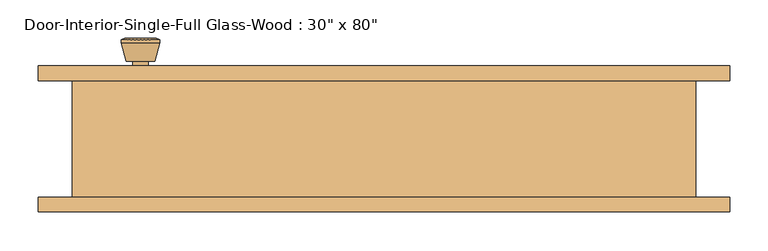
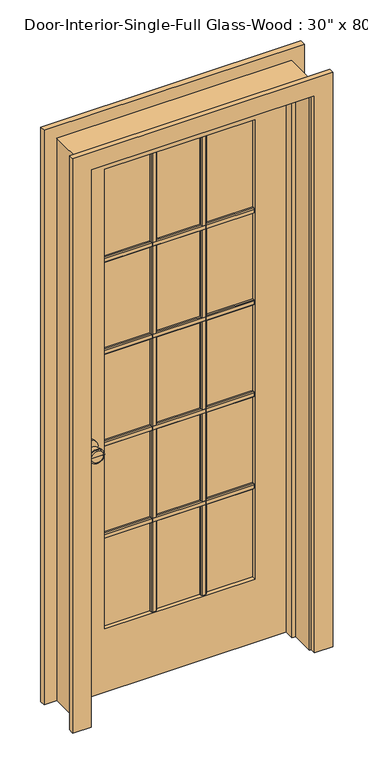
"""IFC4 building model written with IfcOpenShell, lengths in millimetres: door geometry."""

from ifc_helpers import new_model, si_unit, point, frame, frame_2d, origin, place, context, project, spatial, polyline, circle_curve, trimmed, segment, composite_curve, outline, extrude, faceted_brep, source, transform, mapped, element, save
from ifc_brep_helpers import plane_surface, cylinder_surface, revolved_surface, advanced_brep


def door_fa41f557(model_context):
    return source(origin(), model_context, "Body", "SolidModel", [
        extrude(outline(polyline([(59.055, 1586.23), (65.405, 1586.23), (68.58, 1583.055), (68.58, 1570.355), (65.405, 1567.18), (59.055, 1567.18), (59.055, 1586.23)])), frame((-260.35, 0.0, 0.0), z_axis=(1.0, 0.0, 0.0), x_axis=(0.0, 1.0, 0.0)), (0.0, 0.0, 1.0), 520.7),
        extrude(outline(polyline([(59.055, 1249.9975), (65.405, 1249.9975), (68.58, 1246.8225), (68.58, 1234.1225), (65.405, 1230.9475), (59.055, 1230.9475), (59.055, 1249.9975)])), frame((-260.35, 0.0, 0.0), z_axis=(1.0, 0.0, 0.0), x_axis=(0.0, 1.0, 0.0)), (0.0, 0.0, 1.0), 520.7),
        extrude(outline(polyline([(59.055, 913.765), (65.405, 913.765), (68.58, 910.59), (68.58, 897.89), (65.405, 894.715), (59.055, 894.715), (59.055, 913.765)])), frame((-260.35, 0.0, 0.0), z_axis=(1.0, 0.0, 0.0), x_axis=(0.0, 1.0, 0.0)), (0.0, 0.0, 1.0), 520.7),
        extrude(outline(polyline([(59.055, 577.5325), (65.405, 577.5325), (68.58, 574.3575), (68.58, 561.6575), (65.405, 558.4825), (59.055, 558.4825), (59.055, 577.5325)])), frame((-260.35, 0.0, 0.0), z_axis=(1.0, 0.0, 0.0), x_axis=(0.0, 1.0, 0.0)), (0.0, 0.0, 1.0), 520.7),
        extrude(outline(polyline([(77.2583333, 59.055), (77.2583333, 65.405), (80.4333333, 68.58), (93.1333333, 68.58), (96.3083333, 65.405), (96.3083333, 59.055), (77.2583333, 59.055)])), frame((0.0, 0.0, 231.775), z_axis=(0.0, 0.0, 1.0), x_axis=(1.0, 0.0, 0.0)), (0.0, 0.0, 1.0), 1681.1625),
        extrude(outline(polyline([(-96.3083333, 59.055), (-96.3083333, 65.405), (-93.1333333, 68.58), (-80.4333333, 68.58), (-77.2583333, 65.405), (-77.2583333, 59.055), (-96.3083333, 59.055)])), frame((0.0, 0.0, 231.775), z_axis=(0.0, 0.0, 1.0), x_axis=(1.0, 0.0, 0.0)), (0.0, 0.0, 1.0), 1681.1625),
        extrude(outline(polyline([(52.07, 1586.23), (52.07, 1567.18), (45.72, 1567.18), (42.545, 1570.355), (42.545, 1583.055), (45.72, 1586.23), (52.07, 1586.23)])), frame((-260.35, 0.0, 0.0), z_axis=(1.0, 0.0, 0.0), x_axis=(0.0, 1.0, 0.0)), (0.0, 0.0, 1.0), 520.7),
        extrude(outline(polyline([(52.07, 1249.9975), (52.07, 1230.9475), (45.72, 1230.9475), (42.545, 1234.1225), (42.545, 1246.8225), (45.72, 1249.9975), (52.07, 1249.9975)])), frame((-260.35, 0.0, 0.0), z_axis=(1.0, 0.0, 0.0), x_axis=(0.0, 1.0, 0.0)), (0.0, 0.0, 1.0), 520.7),
        extrude(outline(polyline([(52.07, 913.765), (52.07, 894.715), (45.72, 894.715), (42.545, 897.89), (42.545, 910.59), (45.72, 913.765), (52.07, 913.765)])), frame((-260.35, 0.0, 0.0), z_axis=(1.0, 0.0, 0.0), x_axis=(0.0, 1.0, 0.0)), (0.0, 0.0, 1.0), 520.7),
        extrude(outline(polyline([(52.07, 577.5325), (52.07, 558.4825), (45.72, 558.4825), (42.545, 561.6575), (42.545, 574.3575), (45.72, 577.5325), (52.07, 577.5325)])), frame((-260.35, 0.0, 0.0), z_axis=(1.0, 0.0, 0.0), x_axis=(0.0, 1.0, 0.0)), (0.0, 0.0, 1.0), 520.7),
        extrude(outline(polyline([(77.2583333, 52.07), (96.3083333, 52.07), (96.3083333, 45.72), (93.1333333, 42.545), (80.4333333, 42.545), (77.2583333, 45.72), (77.2583333, 52.07)])), frame((0.0, 0.0, 231.775), z_axis=(0.0, 0.0, 1.0), x_axis=(1.0, 0.0, 0.0)), (0.0, 0.0, 1.0), 1681.1625),
        extrude(outline(polyline([(-96.3083333, 52.07), (-77.2583333, 52.07), (-77.2583333, 45.72), (-80.4333333, 42.545), (-93.1333333, 42.545), (-96.3083333, 45.72), (-96.3083333, 52.07)])), frame((0.0, 0.0, 231.775), z_axis=(0.0, 0.0, 1.0), x_axis=(1.0, 0.0, 0.0)), (0.0, 0.0, 1.0), 1681.1625),
        advanced_brep(
        [(-317.5, 32.1, 914.4), (-307.5, 32.1, 914.4), (-327.5, 32.1, 914.4), (-297.0241324, -16.9, 914.4), (-317.5, -16.9, 914.4), (-337.9758676, -16.9, 914.4), (-292.5, -15.0721319, 914.4), (-342.5, -15.0721319, 914.4), (-292.5, -11.6084537, 914.4), (-342.5, -11.6084537, 914.4), (-298.863764, 13.1, 914.4), (-336.136236, 13.1, 914.4), (-307.5, 13.1, 914.4), (-327.5, 13.1, 914.4)],
        [
            (0, 1),
            (1, 2, circle_curve(frame((-317.5, 32.1, 914.4), z_axis=(0.0, 1.0, 0.0), x_axis=(-1.0, 0.0, 0.0)), 10.0)),
            (2, 0),
            (2, 1, circle_curve(frame((-317.5, 32.1, 914.4), z_axis=(0.0, 1.0, 0.0), x_axis=(-1.0, 0.0, 0.0)), 10.0)),
            (3, 4),
            (4, 5),
            (5, 3, circle_curve(frame((-317.5, -16.9, 914.4), z_axis=(0.0, -1.0, 0.0), x_axis=(-1.0, 0.0, 0.0)), 20.4758676)),
            (3, 5, circle_curve(frame((-317.5, -16.9, 914.4), z_axis=(0.0, -1.0, 0.0), x_axis=(-1.0, 0.0, 0.0)), 20.4758676)),
            (6, 3),
            (5, 7),
            (7, 6, circle_curve(frame((-317.5, -15.0721319, 914.4), z_axis=(0.0, -1.0, 0.0), x_axis=(-1.0, 0.0, 0.0)), 25.0)),
            (6, 7, circle_curve(frame((-317.5, -15.0721319, 914.4), z_axis=(0.0, -1.0, 0.0), x_axis=(-1.0, 0.0, 0.0)), 25.0)),
            (8, 6),
            (7, 9),
            (9, 8, circle_curve(frame((-317.5, -11.6084537, 914.4), z_axis=(0.0, -1.0, 0.0), x_axis=(-1.0, 0.0, 0.0)), 25.0)),
            (8, 9, circle_curve(frame((-317.5, -11.6084537, 914.4), z_axis=(0.0, -1.0, 0.0), x_axis=(-1.0, 0.0, 0.0)), 25.0)),
            (10, 8),
            (9, 11),
            (11, 10, circle_curve(frame((-317.5, 13.1, 914.4), z_axis=(0.0, -1.0, 0.0), x_axis=(-1.0, 0.0, 0.0)), 18.636236)),
            (10, 11, circle_curve(frame((-317.5, 13.1, 914.4), z_axis=(0.0, -1.0, 0.0), x_axis=(-1.0, 0.0, 0.0)), 18.636236)),
            (12, 10),
            (11, 13),
            (13, 12, circle_curve(frame((-317.5, 13.1, 914.4), z_axis=(0.0, -1.0, 0.0), x_axis=(-1.0, 0.0, 0.0)), 10.0)),
            (12, 13, circle_curve(frame((-317.5, 13.1, 914.4), z_axis=(0.0, -1.0, 0.0), x_axis=(-1.0, 0.0, 0.0)), 10.0)),
            (1, 12),
            (13, 2),
        ],
        [
            plane_surface(frame((-317.5, 32.1, 914.4), z_axis=(0.0, 1.0, 0.0), x_axis=(-1.0, 0.0, 0.0))),
            plane_surface(frame((-317.5, -16.9, 914.4), z_axis=(0.0, -1.0, 0.0), x_axis=(-1.0, 0.0, 0.0))),
            revolved_surface(polyline([(-337.9758676, -16.9, 914.4), (-342.5, -15.0721319, 914.4)]), (-317.5, 32.1, 914.4), (0.0, 1.0, 0.0)),
            cylinder_surface(frame((-317.5, 32.1, 914.4), z_axis=(0.0, 1.0, 0.0), x_axis=(-1.0, 0.0, 0.0)), 25.0),
            revolved_surface(polyline([(-342.5, -11.6084537, 914.4), (-336.136236, 13.1, 914.4)]), (-317.5, 32.1, 914.4), (0.0, 1.0, 0.0)),
            plane_surface(frame((-317.5, 13.1, 914.4), z_axis=(0.0, 1.0, 0.0), x_axis=(-1.0, 0.0, 0.0))),
            cylinder_surface(frame((-317.5, 32.1, 914.4), z_axis=(0.0, 1.0, 0.0), x_axis=(-1.0, 0.0, 0.0)), 10.0),
        ],
        [
            (0, [[1, 2, 3]]),
            (0, [[-3, 4, -1]]),
            (1, [[5, 6, 7]]),
            (1, [[-6, -5, 8]]),
            (2, [[9, -7, 10, 11]]),
            (2, [[-10, -8, -9, 12]]),
            (3, [[13, -11, 14, 15]]),
            (3, [[-14, -12, -13, 16]]),
            (4, [[17, -15, 18, 19]]),
            (4, [[-18, -16, -17, 20]]),
            (5, [[21, -19, 22, 23]]),
            (5, [[-22, -20, -21, 24]]),
            (6, [[25, -23, 26, -2]]),
            (6, [[-26, -24, -25, -4]]),
        ],
    ),
        extrude(outline(composite_curve([segment(trimmed(circle_curve(frame_2d((914.4, -317.5)), 30.0), [point((914.4, -347.5))], [point((914.4, -287.5))], False, "CARTESIAN"), True, "CONTINUOUS"), segment(trimmed(circle_curve(frame_2d((914.4, -317.5)), 30.0), [point((914.4, -287.5))], [point((914.4, -347.5))], False, "CARTESIAN"), True, "CONTINUOUS")], self_intersect=False)), frame((0.0, 32.1, 0.0), z_axis=(0.0, 1.0, 0.0), x_axis=(0.0, 0.0, 1.0)), (0.0, 0.0, 1.0), 6.0),
        advanced_brep(
        [(-317.5, 79.025, 914.4), (-327.5, 79.025, 914.4), (-307.5, 79.025, 914.4), (-297.0241324, 128.025, 914.4), (-337.9758676, 128.025, 914.4), (-317.5, 128.025, 914.4), (-292.5, 126.1971319, 914.4), (-342.5, 126.1971319, 914.4), (-292.5, 122.7334537, 914.4), (-342.5, 122.7334537, 914.4), (-298.863764, 98.025, 914.4), (-336.136236, 98.025, 914.4), (-307.5, 98.025, 914.4), (-327.5, 98.025, 914.4)],
        [
            (0, 1),
            (1, 2, circle_curve(frame((-317.5, 79.025, 914.4), z_axis=(0.0, -1.0, 0.0), x_axis=(-1.0, 0.0, 0.0)), 10.0)),
            (2, 0),
            (2, 1, circle_curve(frame((-317.5, 79.025, 914.4), z_axis=(0.0, -1.0, 0.0), x_axis=(-1.0, 0.0, 0.0)), 10.0)),
            (3, 4, circle_curve(frame((-317.5, 128.025, 914.4), z_axis=(0.0, 1.0, 0.0), x_axis=(-1.0, 0.0, 0.0)), 20.4758676)),
            (4, 5),
            (5, 3),
            (4, 3, circle_curve(frame((-317.5, 128.025, 914.4), z_axis=(0.0, 1.0, 0.0), x_axis=(-1.0, 0.0, 0.0)), 20.4758676)),
            (6, 7, circle_curve(frame((-317.5, 126.1971319, 914.4), z_axis=(0.0, 1.0, 0.0), x_axis=(-1.0, 0.0, 0.0)), 25.0)),
            (7, 4),
            (3, 6),
            (7, 6, circle_curve(frame((-317.5, 126.1971319, 914.4), z_axis=(0.0, 1.0, 0.0), x_axis=(-1.0, 0.0, 0.0)), 25.0)),
            (8, 9, circle_curve(frame((-317.5, 122.7334537, 914.4), z_axis=(0.0, 1.0, 0.0), x_axis=(-1.0, 0.0, 0.0)), 25.0)),
            (9, 7),
            (6, 8),
            (9, 8, circle_curve(frame((-317.5, 122.7334537, 914.4), z_axis=(0.0, 1.0, 0.0), x_axis=(-1.0, 0.0, 0.0)), 25.0)),
            (10, 11, circle_curve(frame((-317.5, 98.025, 914.4), z_axis=(0.0, 1.0, 0.0), x_axis=(-1.0, 0.0, 0.0)), 18.636236)),
            (11, 9),
            (8, 10),
            (11, 10, circle_curve(frame((-317.5, 98.025, 914.4), z_axis=(0.0, 1.0, 0.0), x_axis=(-1.0, 0.0, 0.0)), 18.636236)),
            (12, 13, circle_curve(frame((-317.5, 98.025, 914.4), z_axis=(0.0, 1.0, 0.0), x_axis=(-1.0, 0.0, 0.0)), 10.0)),
            (13, 11),
            (10, 12),
            (13, 12, circle_curve(frame((-317.5, 98.025, 914.4), z_axis=(0.0, 1.0, 0.0), x_axis=(-1.0, 0.0, 0.0)), 10.0)),
            (1, 13),
            (12, 2),
        ],
        [
            plane_surface(frame((-317.5, 79.025, 914.4), z_axis=(0.0, -1.0, 0.0), x_axis=(-1.0, 0.0, 0.0))),
            plane_surface(frame((-317.5, 128.025, 914.4), z_axis=(0.0, 1.0, 0.0), x_axis=(-1.0, 0.0, 0.0))),
            revolved_surface(polyline([(-337.9758676, 128.025, 914.4), (-342.5, 126.1971319, 914.4)]), (-317.5, 79.025, 914.4), (0.0, -1.0, 0.0)),
            cylinder_surface(frame((-317.5, 79.025, 914.4), z_axis=(0.0, -1.0, 0.0), x_axis=(-1.0, 0.0, 0.0)), 25.0),
            revolved_surface(polyline([(-342.5, 122.7334537, 914.4), (-336.136236, 98.025, 914.4)]), (-317.5, 79.025, 914.4), (0.0, -1.0, 0.0)),
            plane_surface(frame((-317.5, 98.025, 914.4), z_axis=(0.0, -1.0, 0.0), x_axis=(-1.0, 0.0, 0.0))),
            cylinder_surface(frame((-317.5, 79.025, 914.4), z_axis=(0.0, -1.0, 0.0), x_axis=(-1.0, 0.0, 0.0)), 10.0),
        ],
        [
            (0, [[1, 2, 3]]),
            (0, [[-3, 4, -1]]),
            (1, [[5, 6, 7]]),
            (1, [[8, -7, -6]]),
            (2, [[9, 10, -5, 11]]),
            (2, [[12, -11, -8, -10]]),
            (3, [[13, 14, -9, 15]]),
            (3, [[16, -15, -12, -14]]),
            (4, [[17, 18, -13, 19]]),
            (4, [[20, -19, -16, -18]]),
            (5, [[21, 22, -17, 23]]),
            (5, [[24, -23, -20, -22]]),
            (6, [[-2, 25, -21, 26]]),
            (6, [[-4, -26, -24, -25]]),
        ],
    ),
        extrude(outline(composite_curve([segment(trimmed(circle_curve(frame_2d((914.4, -317.5)), 30.0), [point((914.4, -347.5))], [point((914.4, -287.5))], False, "CARTESIAN"), True, "CONTINUOUS"), segment(trimmed(circle_curve(frame_2d((914.4, -317.5)), 30.0), [point((914.4, -287.5))], [point((914.4, -347.5))], False, "CARTESIAN"), True, "CONTINUOUS")], self_intersect=False)), frame((0.0, 73.025, 0.0), z_axis=(0.0, 1.0, 0.0), x_axis=(0.0, 0.0, 1.0)), (0.0, 0.0, 1.0), 6.0),
        extrude(outline(polyline([(2032.0, -381.0), (0.0, -381.0), (0.0, 381.0), (2032.0, 381.0), (2032.0, -381.0)]), holes=[polyline([(1912.9375, -260.35), (1912.9375, 260.35), (231.775, 260.35), (231.775, -260.35), (1912.9375, -260.35)])]), frame((0.0, 38.1, 0.0), z_axis=(0.0, 1.0, 0.0), x_axis=(0.0, 0.0, 1.0)), (0.0, 0.0, 1.0), 34.925),
        faceted_brep([(406.4, 73.025, 0.0), (406.4, -79.375, 0.0), (381.0, -79.375, 0.0), (381.0, 3.175, 0.0), (368.3, 3.175, 0.0), (368.3, 38.1, 0.0), (381.0, 38.1, 0.0), (381.0, 73.025, 0.0), (406.4, 73.025, 2057.4), (406.4, -79.375, 2057.4), (-406.4, -79.375, 2057.4), (-406.4, -79.375, 0.0), (-381.0, -79.375, 0.0), (-381.0, -79.375, 2032.0), (381.0, -79.375, 2032.0), (381.0, 3.175, 2032.0), (-381.0, 3.175, 2032.0), (-381.0, 3.175, 0.0), (-368.3, 3.175, 0.0), (-368.3, 3.175, 2019.3), (368.3, 3.175, 2019.3), (368.3, 38.1, 2019.3), (-368.3, 38.1, 2019.3), (-368.3, 38.1, 0.0), (-381.0, 38.1, 0.0), (-381.0, 38.1, 2032.0), (381.0, 38.1, 2032.0), (381.0, 73.025, 2032.0), (-381.0, 73.025, 2032.0), (-381.0, 73.025, 0.0), (-406.4, 73.025, 0.0), (-406.4, 73.025, 2057.4)], [[[0, 1, 2, 3, 4, 5, 6, 7]], [[1, 0, 8, 9]], [[2, 1, 9, 10, 11, 12, 13, 14]], [[3, 2, 14, 15]], [[4, 3, 15, 16, 17, 18, 19, 20]], [[5, 4, 20, 21]], [[6, 5, 21, 22, 23, 24, 25, 26]], [[7, 6, 26, 27]], [[0, 7, 27, 28, 29, 30, 31, 8]], [[9, 8, 31, 10]], [[15, 14, 13, 16]], [[21, 20, 19, 22]], [[27, 26, 25, 28]], [[30, 29, 24, 23, 18, 17, 12, 11]], [[10, 31, 30, 11]], [[16, 13, 12, 17]], [[22, 19, 18, 23]], [[28, 25, 24, 29]]]),
        extrude(outline(polyline([(260.35, 52.07), (-260.35, 52.07), (-260.35, 59.055), (260.35, 59.055), (260.35, 52.07)])), frame((0.0, 0.0, 231.775), z_axis=(0.0, 0.0, 1.0), x_axis=(1.0, 0.0, 0.0)), (0.0, 0.0, 1.0), 1681.1625),
        extrude(outline(polyline([(0.0, 387.35), (0.0, 450.85), (2101.85, 450.85), (2101.85, -450.85), (0.0, -450.85), (0.0, -387.35), (2038.35, -387.35), (2038.35, 387.35), (0.0, 387.35)])), frame((0.0, -98.425, 0.0), z_axis=(0.0, 1.0, 0.0), x_axis=(0.0, 0.0, 1.0)), (0.0, 0.0, 1.0), 19.05),
        extrude(outline(polyline([(0.0, 387.35), (0.0, 450.85), (2101.85, 450.85), (2101.85, -450.85), (0.0, -450.85), (0.0, -387.35), (2038.35, -387.35), (2038.35, 387.35), (0.0, 387.35)])), frame((0.0, 73.025, 0.0), z_axis=(0.0, 1.0, 0.0), x_axis=(0.0, 0.0, 1.0)), (0.0, 0.0, 1.0), 19.05),
    ])


if __name__ == "__main__":
    model = new_model("IFC4")
    model_context = context("Model", 3, world=origin())
    ifc_project = project(units=[si_unit("LENGTHUNIT", "METRE", prefix="MILLI")], contexts=[model_context])
    site = spatial("IfcSite", under=ifc_project)
    building = spatial("IfcBuilding", under=site)
    placement = place(None, origin())
    door_shape = door_fa41f557(model_context)
    element("IfcDoor", 1, ObjectType="Door-Interior-Single-Full Glass-Wood : 30\" x 80\"", at=placement, inside=building, context=model_context, shape_type="MappedRepresentation", body=[
        mapped(door_shape, transform((0.0, 0.0, 0.0), x_axis=(1.0, 0.0, 0.0), y_axis=(0.0, 1.0, 0.0), z_axis=(0.0, 0.0, 1.0))),
    ])
    save(model, "model.ifc")

# Revit data of these elements
# Type "Door-Interior-Single-Full Glass-Wood : 30\" x 80\""
#   Type Mark = "10"
#   Assembly Code = "C1020300"
#   Analytic Construction = "Wood frame with single clear glass"
#   Top Rail = 0' - 4 11/16"
#   Thickness = 0' - 1 3/8"
#   Thermal Resistance (R) = 1.0102 (h·ft²·°F)/BTU
#   Swing Angle [instance default] = 90.00°
#   Stiles = 0' - 4 3/4"
#   Rough Width = 2' - 8"
#   Rough Height = 6' - 9"
#   Height = 6' - 8"
#   Width = 2' - 6"
#   Heat Transfer Coefficient (U) = 0.9900 BTU/(h·ft²·°F)
#   Bottom Rail = 0' - 9 1/8"
#   Show Grill [instance default] = yes
#   Trim Material = Cherry
#   Panel Material = Cherry
#   Frame Material = Cherry
#   Door Handle Material = Aluminum
#   Visual Light Transmittance = 0
#   Solar Heat Gain Coefficient = 0
#   Wall Closure = (empty or 0)
#   Function = (empty or 0)
# Element 1 (IfcDoor, "Door-Interior-Single-Full Glass-Wood : 30\" x 80\"")
#   Materials on its faces: "Cherry", "Aluminum", "Glass"
# Materials
#   "Cherry": class "Wood", colour RGB 226 177 128, transparency 0, Description = "Prunus Serotina", Cost = 0
#   "Aluminum": class "Metal", colour RGB 247 247 247, transparency 0, Description = "Aluminum 6061", Cost = 0
#   "Glass": class "Glass", colour RGB 0 128 192, transparency 0.75, Description = "Soda Lime Glass", Cost = 0
